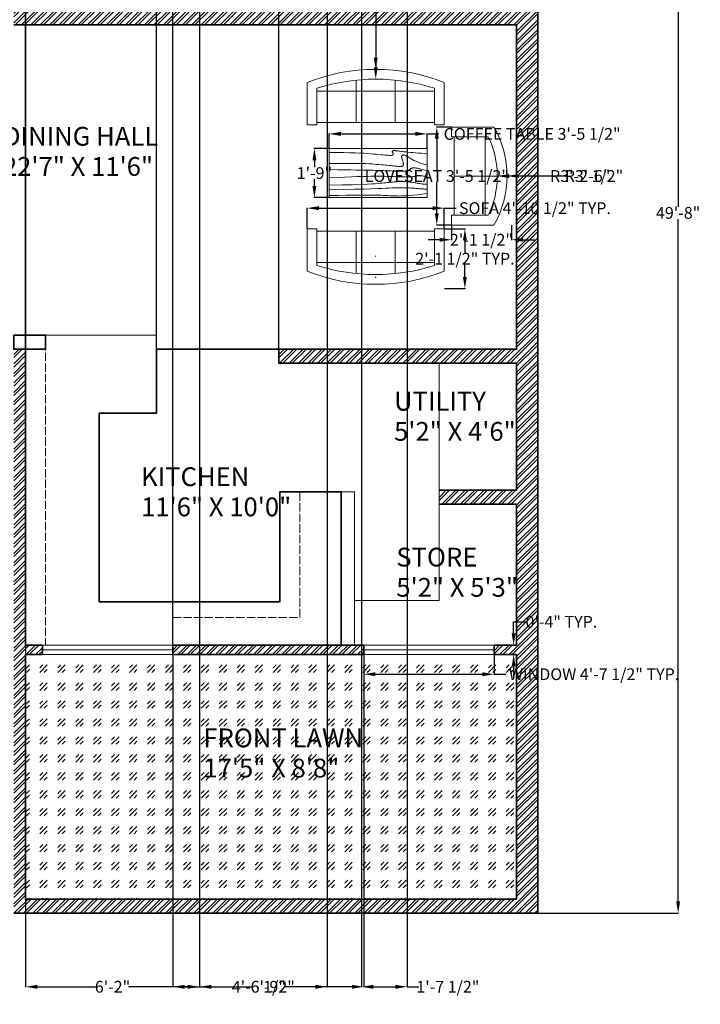
# Model space of a CAD drawing. Units: inches. Extents: x 334 to 846, y -424 to 250.
# Tile 2 of 3: x 557 to 846, y -424 to -5. Entities that reach past the tile are written whole.
import ezdxf

# ---------------------------------------------------------------- set-up
doc = ezdxf.new("R2010")
doc.units = ezdxf.units.IN
doc.header["$MEASUREMENT"] = 0
doc.linetypes.add('ACAD_ISO02W100', pattern=[15, 12, -3])
for name, color, linetype, lineweight in [('A-AREA-IDEN', 130, 'Continuous', 18), ('A-FLOR-FIXT', 8, 'Continuous', 18), ('A-FLOR-FIXT-HIDN', 8, 'ACAD_ISO02W100', 13), ('A-WALL', 7, 'Continuous', 35), ('A-WALL-PATT', 252, 'Continuous', 13), ('dimension', 130, 'Continuous', 18), ('furniture', 6, 'Continuous', 18), ('L-PLNT-PATT', 114, 'Continuous', 13), ('window', 150, 'Continuous', 18)]:
    doc.layers.add(name, color=color, linetype=linetype, lineweight=lineweight)
doc.styles.get("Standard").update_dxf_attribs({"font": 'arial.ttf'})
doc.dimstyles.get("Standard").update_dxf_attribs({"dimtxt": 5, "dimasz": 5, "dimexe": 0.18, "dimexo": 0.0625, "dimgap": 0.09, "dimtad": 0, "dimtih": 1, "dimtoh": 1, "dimdec": 1, "dimzin": 0, "dimdsep": 46, "dimlunit": 4, "dimtxsty": 'Standard', "dimcen": 0.09, "dimadec": 0, "dimazin": 0, "dimtfac": 1, "dimtdec": 1, "dimtofl": 0, "dimtmove": 0, "dimatfit": 3, "dimfxl": 1, "dimtolj": 1, "dimtzin": 0, "dimarcsym": 0})

# ---------------------------------------------------------------- blocks, each defined once
blk = doc.blocks.new('Sofa - Roundback 7 ft.')
for p, q in [((-36.000027, -34), (-36.000027, -11.4696)), ((-12.00002, -32.4421), (-12.00003, -6.5971)), ((11.99997, -32.4421), (11.99998, -6.5971)), ((35.99998, -34), (35.99998, -11.4696)), ((-35.999844, -13.3819), (35.9998, -13.3819)), ((-36.000027, -32.4421), (35.99998, -32.4421))]:
    blk.add_line(p, q)
for points in [[(-36.000027, -34), (-42.000027, -34), (-42.000027, -8)], [(41.99998, -8), (41.99998, -34), (35.99998, -34)]]:
    blk.add_lwpolyline(points)
for centre, radius, start, end in [((0, -114.25), 114.25, 68.43141, 111.5686), ((-0.00001, -127.1968), 121.1968, 72.72033, 107.2797)]:
    blk.add_arc(centre, radius, start, end)
blk = doc.blocks.new('Sofa - Roundback Loveseat 5 ft.')
for p, q in [((0, -32.44198), (0, -5.99998)), ((-24, -33.99998), (-24, -11.46958)), ((24.00004, -33.99998), (24.00004, -11.46958)), ((-23.9998, -13.38178), (23.99986, -13.38178)), ((-24, -32.44198), (24.00004, -32.44198))]:
    blk.add_line(p, q)
for points in [[(-24, -33.99998), (-30, -33.99998), (-30, -7.99998)], [(30.00004, -7.99998), (30.00004, -33.99998), (24.00004, -33.99998)]]:
    blk.add_lwpolyline(points)
for centre, radius, start, end in [((0, -60.24998), 60.24998, 60.13715, 119.8628), ((0, -61.38438), 55.38444, 64.32083, 115.6792)]:
    blk.add_arc(centre, radius, start, end)
blk = doc.blocks.new('Table - Rectangular Woodgrain 60 x 30 in.')
for p, q in [((0, 0), (0, -30)), ((60, 0), (0, 0)), ((60, -30), (60, 0)), ((0, -30), (60, -30))]:
    blk.add_line(p, q)
for points in [[(0, -2.4), (4.8155, -2.418), (9.0302, -2.4688), (12.709, -2.5477), (15.9167, -2.65), (18.7181, -2.7711), (21.1781, -2.9063), (23.3616, -3.0508), (25.3333, -3.2), (27.1477, -3.3495), (28.8172, -3.4958), (30.3437, -3.636), (31.7291, -3.7667), (32.9756, -3.8849), (34.0849, -3.9875), (35.059, -4.0714), (35.9, -4.1334), (36.6114, -4.1711), (37.2041, -4.1854), (37.6906, -4.1779), (38.0833, -4.15), (38.3948, -4.1034), (38.6375, -4.0396), (38.8239, -3.9602), (38.9666, -3.8667), (39.0764, -3.7608), (39.1573, -3.6448), (39.2116, -3.521), (39.2416, -3.3917), (39.2498, -3.2593), (39.2385, -3.1261), (39.21, -2.9944), (39.1666, -2.8667), (39.111, -2.7447), (39.0468, -2.6281), (38.978, -2.5163), (38.9083, -2.4083), (38.8418, -2.3035), (38.7823, -2.201), (38.7337, -2.1001), (38.7, -2), (38.6844, -1.9003), (38.6875, -1.8021), (38.7094, -1.707), (38.75, -1.6167), (38.8094, -1.5326), (38.8875, -1.4563), (38.9844, -1.3893), (39.1, -1.3333), (39.2351, -1.2896), (39.3937, -1.2583), (39.5804, -1.2396), (39.8, -1.2333), (40.057, -1.2396), (40.3562, -1.2583), (40.7023, -1.2896), (41.1, -1.3333), (41.5547, -1.3895), (42.0755, -1.4573), (42.6721, -1.5361), (43.3542, -1.625), (44.1316, -1.7233), (45.014, -1.8302), (46.0114, -1.9449), (47.1333, -2.0667), (48.3862, -2.1947), (49.7625, -2.3281), (51.2513, -2.4663), (52.8416, -2.6083), (54.5226, -2.7535), (56.2833, -2.9011), (58.1127, -3.0501), (60, -3.2)], [(0, -9.2), (6.5759, -9.0858), (11.9385, -9.0365), (16.2527, -9.0418), (19.6833, -9.0917), (22.3952, -9.1759), (24.5531, -9.2844), (26.322, -9.4069), (27.8666, -9.5333), (29.3241, -9.6553), (30.7203, -9.7719), (32.0532, -9.8837), (33.3208, -9.9917), (34.5213, -10.0965), (35.6526, -10.199), (36.7128, -10.2999), (37.7, -10.4), (38.6129, -10.4996), (39.4531, -10.5969), (40.223, -10.6895), (40.925, -10.775), (41.5613, -10.8512), (42.1344, -10.9156), (42.6465, -10.966), (43.1, -11), (43.4976, -11.0158), (43.8437, -11.0136), (44.143, -10.9942), (44.4, -10.9583), (44.6195, -10.9069), (44.8062, -10.8406), (44.9648, -10.7603), (45.1, -10.6667), (45.2155, -10.5598), (45.3114, -10.4365), (45.3871, -10.2929), (45.4416, -10.125), (45.4743, -9.929), (45.4844, -9.7011), (45.4709, -9.4371), (45.4333, -9.1333), (45.3716, -8.7883), (45.2896, -8.4104), (45.1919, -8.0107), (45.0833, -7.6), (44.9685, -7.1893), (44.8521, -6.7896), (44.7388, -6.4117), (44.6333, -6.0667), (44.54, -5.7628), (44.4614, -5.4979), (44.4001, -5.2675), (44.3583, -5.0667), (44.3384, -4.8909), (44.3427, -4.7354), (44.3736, -4.5956), (44.4333, -4.4667), (44.5236, -4.3453), (44.6427, -4.2333), (44.7884, -4.1339), (44.9583, -4.05), (45.1501, -3.9849), (45.3614, -3.9417), (45.59, -3.9234), (45.8333, -3.9333), (46.0915, -3.9749), (46.3734, -4.0531), (46.6906, -4.1736), (47.0542, -4.3417), (47.4756, -4.5629), (47.9661, -4.8427), (48.5372, -5.1866), (49.2, -5.6), (49.9676, -6.0844), (50.8594, -6.625), (51.8965, -7.2031), (53.1, -7.8), (54.491, -8.3969), (56.0906, -8.975), (57.9199, -9.5156), (60, -10)], [(0, -12.8), (5.1847, -12.9322), (9.6213, -13.0323), (13.3963, -13.1059), (16.5958, -13.1583), (19.3063, -13.1952), (21.614, -13.2219), (23.6054, -13.2439), (25.3666, -13.2667), (26.9728, -13.2947), (28.4531, -13.3281), (29.8256, -13.3663), (31.1083, -13.4083), (32.3191, -13.4535), (33.476, -13.501), (34.597, -13.5501), (35.7, -13.6), (36.7984, -13.6497), (37.8875, -13.6979), (38.9578, -13.743), (40, -13.7833), (41.0047, -13.8174), (41.9625, -13.8438), (42.864, -13.8607), (43.7, -13.8667), (44.4631, -13.8604), (45.1552, -13.8417), (45.7801, -13.8104), (46.3416, -13.7667), (46.8439, -13.7104), (47.2906, -13.6417), (47.6858, -13.5604), (48.0333, -13.4667), (48.3375, -13.3608), (48.6042, -13.2448), (48.8396, -13.121), (49.05, -12.9917), (49.2417, -12.8593), (49.4208, -12.7261), (49.5937, -12.5944), (49.7667, -12.4667), (49.9452, -12.3451), (50.1323, -12.2313), (50.3303, -12.1268), (50.5416, -12.0333), (50.7686, -11.9524), (51.0135, -11.8854), (51.2788, -11.8341), (51.5666, -11.8), (51.8785, -11.7843), (52.2116, -11.7865), (52.562, -11.8059), (52.926, -11.8417), (53.2998, -11.8931), (53.6795, -11.9594), (54.0614, -12.0397), (54.4416, -12.1333), (54.8223, -12.2401), (55.2293, -12.3625), (55.6942, -12.5037), (56.2489, -12.6667), (56.9251, -12.8547), (57.7545, -13.0708), (58.7689, -13.3182), (60, -13.6)], [(0, -18), (5.124, -17.7273), (9.6609, -17.5057), (13.6705, -17.3303), (17.2125, -17.1958), (20.3467, -17.0973), (23.1328, -17.0297), (25.6307, -16.9878), (27.9, -16.9667), (29.9928, -16.9617), (31.9302, -16.9703), (33.7254, -16.9907), (35.3917, -17.0208), (36.9423, -17.0588), (38.3906, -17.1026), (39.7499, -17.1503), (41.0333, -17.2), (42.2519, -17.2496), (43.4073, -17.2969), (44.4986, -17.3395), (45.525, -17.375), (46.4858, -17.4012), (47.3802, -17.4156), (48.2074, -17.416), (48.9667, -17.4), (49.6583, -17.3662), (50.2872, -17.3167), (50.8595, -17.2547), (51.3812, -17.1833), (51.8584, -17.1057), (52.2971, -17.025), (52.7034, -16.9443), (53.0833, -16.8667), (53.443, -16.7951), (53.789, -16.7313), (54.128, -16.6768), (54.4666, -16.6334), (54.8115, -16.6024), (55.1693, -16.5854), (55.5465, -16.5841), (55.95, -16.6), (56.3828, -16.6337), (56.8346, -16.6823), (57.2915, -16.7418), (57.7396, -16.8084), (58.165, -16.878), (58.5539, -16.9469), (58.8924, -17.0111), (59.1666, -17.0667), (59.3679, -17.1107), (59.5078, -17.1438), (59.6032, -17.1675), (59.6708, -17.1833), (59.7275, -17.193), (59.7901, -17.1979), (59.8753, -17.1998), (60, -17.2)], [(0, -22.4), (8.0098, -22.2501), (14.4094, -22.1011), (19.4168, -21.9535), (23.25, -21.8083), (26.1269, -21.6663), (28.2656, -21.5281), (29.884, -21.3947), (31.2, -21.2667), (32.3967, -21.1448), (33.5172, -21.0292), (34.5697, -20.9198), (35.5625, -20.8167), (36.5037, -20.7198), (37.4015, -20.6292), (38.2642, -20.5448), (39.1, -20.4667), (39.9164, -20.3951), (40.7187, -20.3313), (41.5117, -20.2768), (42.3, -20.2333), (43.0883, -20.2024), (43.8812, -20.1854), (44.6836, -20.1841), (45.5, -20.2), (46.3328, -20.234), (47.1747, -20.2844), (48.0163, -20.3488), (48.8479, -20.425), (49.66, -20.5106), (50.4429, -20.6031), (51.1872, -20.7004), (51.8833, -20.8), (52.5246, -20.8999), (53.1166, -20.9995), (53.6681, -21.0983), (54.1875, -21.1958), (54.6834, -21.2919), (55.1646, -21.3859), (55.6394, -21.4777), (56.1167, -21.5667), (56.6028, -21.6515), (57.0961, -21.7266), (57.5929, -21.7852), (58.0896, -21.8208), (58.5823, -21.8268), (59.0674, -21.7964), (59.5412, -21.723), (60, -21.6)], [(0, -25.2), (8.6355, -25.0504), (15.7026, -24.9031), (21.4049, -24.7606), (25.9458, -24.625), (29.529, -24.4988), (32.3578, -24.3844), (34.6359, -24.284), (36.5667, -24.2), (38.3213, -24.1341), (39.9417, -24.0854), (41.437, -24.0523), (42.8167, -24.0333), (44.0901, -24.0268), (45.2667, -24.0313), (46.3557, -24.0451), (47.3667, -24.0667), (48.309, -24.0947), (49.1928, -24.1287), (50.0284, -24.168), (50.826, -24.2125), (51.5959, -24.2617), (52.3483, -24.3151), (53.0935, -24.3725), (53.8417, -24.4334), (54.6009, -24.497), (55.3699, -24.561), (56.1454, -24.6226), (56.9239, -24.6792), (57.7021, -24.7279), (58.4764, -24.7662), (59.2435, -24.7911), (60, -24.8)], [(0, -28.8), (5.6867, -28.6681), (10.45, -28.5698), (14.407, -28.5012), (17.675, -28.4584), (20.3711, -28.4374), (22.6125, -28.4344), (24.5164, -28.4455), (26.2, -28.4667), (27.762, -28.4947), (29.2276, -28.5281), (30.6033, -28.5663), (31.8958, -28.6084), (33.1118, -28.6535), (34.2578, -28.7011), (35.3405, -28.7501), (36.3666, -28.8), (37.3443, -28.8497), (38.288, -28.8974), (39.2137, -28.9412), (40.1375, -28.9792), (41.0753, -29.0093), (42.0432, -29.0297), (43.0572, -29.0384), (44.1333, -29.0333), (45.2936, -29.0114), (46.5843, -28.9641), (48.0579, -28.8816), (49.7666, -28.7542), (51.7629, -28.5721), (54.0989, -28.3255), (56.8272, -28.0048), (60, -27.6)]]:
    blk.add_lwpolyline(points)
blk = doc.blocks.new('*D8')
at = {"layer": 'Defpoints', "color": 0, "ltscale": 0.3, "transparency": 16777216}
for p in [(777.06, 211), (777.06, -385), (836.82, -385)]:
    blk.add_point(p, dxfattribs=at)
at = {"layer": 'dimension', "color": 0, "lineweight": -2, "ltscale": 0.3, "transparency": 16777216}
for p, q in [((777.12, 211), (837, 211)), ((836.82, 206), (836.82, -84.36)), ((836.82, -380), (836.82, -89.65)), ((777.12, -385), (837, -385))]:
    blk.add_line(p, q, dxfattribs=at)
at = {"layer": 'dimension', "color": 0, "ltscale": 0.3, "transparency": 16777216}
for points in [[(835.99, 206), (837.66, 206), (836.82, 211)], [(835.99, -380), (837.66, -380), (836.82, -385)]]:
    blk.add_solid(points, dxfattribs=at)
at = {"layer": 'dimension', "color": 0, "ltscale": 0.3, "transparency": 16777216, "insert": (836.82, -87), "char_height": 5, "attachment_point": 5}
blk.add_mtext('\\A1;49\'-8"', dxfattribs=at)
blk = doc.blocks.new('WIN-55_5IN')
at = {"ltscale": 0.3}
blk.add_line((0, 2), (55.5, 2), dxfattribs=at)
blk.add_lwpolyline([(0, 4), (55.5, 4), (55.5, 0), (0, 0)], close=True, dxfattribs=at)
blk = doc.blocks.new('*D12')
at = {"layer": 'Defpoints', "color": 0, "ltscale": 0.3, "transparency": 16777216}
for p in [(737.3, -84.99), (678.9, -93.75), (737.3, -93.75)]:
    blk.add_point(p, dxfattribs=at)
at = {"layer": 'dimension', "color": 0, "lineweight": -2, "ltscale": 0.3, "transparency": 16777216}
for p, q in [((678.9, -93.69), (678.9, -84.81)), ((683.9, -84.99), (732.3, -84.99)), ((737.3, -93.69), (737.3, -84.81)), ((737.3, -84.99), (742.3, -84.99))]:
    blk.add_line(p, q, dxfattribs=at)
at = {"layer": 'dimension', "color": 0, "ltscale": 0.3, "transparency": 16777216}
for points in [[(683.9, -84.16), (683.9, -85.83), (678.9, -84.99)], [(732.3, -84.16), (732.3, -85.83), (737.3, -84.99)]]:
    blk.add_solid(points, dxfattribs=at)
at = {"layer": 'dimension', "color": 0, "ltscale": 0.3, "transparency": 16777216, "insert": (775.86, -84.99), "char_height": 5, "attachment_point": 5}
blk.add_mtext('\\A1;SOFA 4\'-10 1/2" TYP.', dxfattribs=at)
blk = doc.blocks.new('*D13')
at = {"layer": 'Defpoints', "color": 0, "ltscale": 0.3, "transparency": 16777216}
for p in [(737.3, -93.75), (737.3, -119.24), (746.06, -119.24)]:
    blk.add_point(p, dxfattribs=at)
at = {"layer": 'dimension', "color": 0, "lineweight": -2, "ltscale": 0.3, "transparency": 16777216}
for p, q in [((737.36, -93.75), (746.24, -93.75)), ((746.06, -98.75), (746.06, -103.82)), ((746.06, -114.24), (746.06, -109.17)), ((737.36, -119.24), (746.24, -119.24))]:
    blk.add_line(p, q, dxfattribs=at)
at = {"layer": 'dimension', "color": 0, "ltscale": 0.3, "transparency": 16777216}
for points in [[(745.22, -98.75), (746.89, -98.75), (746.06, -93.75)], [(745.22, -114.24), (746.89, -114.24), (746.06, -119.24)]]:
    blk.add_solid(points, dxfattribs=at)
at = {"layer": 'dimension', "color": 0, "ltscale": 0.3, "transparency": 16777216, "insert": (746.06, -106.5), "char_height": 5, "attachment_point": 5}
blk.add_mtext('\\A1;2\'-1 1/2" TYP.', dxfattribs=at)
blk = doc.blocks.new('*D14')
at = {"layer": 'Defpoints', "color": 0, "ltscale": 0.3, "transparency": 16777216}
for p in [(740.35, -50.46), (734.09, -92.17), (740.35, -92.17)]:
    blk.add_point(p, dxfattribs=at)
at = {"layer": 'dimension', "color": 0, "lineweight": -2, "ltscale": 0.3, "transparency": 16777216}
for p, q in [((740.29, -50.46), (733.91, -50.46)), ((734.09, -55.46), (734.09, -68.64)), ((734.09, -87.17), (734.09, -73.99)), ((740.29, -92.17), (733.91, -92.17))]:
    blk.add_line(p, q, dxfattribs=at)
at = {"layer": 'dimension', "color": 0, "ltscale": 0.3, "transparency": 16777216}
for points in [[(733.26, -55.46), (734.93, -55.46), (734.09, -50.46)], [(733.26, -87.17), (734.93, -87.17), (734.09, -92.17)]]:
    blk.add_solid(points, dxfattribs=at)
at = {"layer": 'dimension', "color": 0, "ltscale": 0.3, "transparency": 16777216, "insert": (734.09, -71.31), "char_height": 5, "attachment_point": 5}
blk.add_mtext('\\A1;LOVESEAT 3\'-5 1/2"', dxfattribs=at)
blk = doc.blocks.new('*D15')
at = {"layer": 'Defpoints', "color": 0, "ltscale": 0.3, "transparency": 16777216}
for p in [(740.35, -92.17), (765.84, -92.17), (765.84, -98.43)]:
    blk.add_point(p, dxfattribs=at)
at = {"layer": 'dimension', "color": 0, "lineweight": -2, "ltscale": 0.3, "transparency": 16777216}
for p, q in [((740.35, -92.23), (740.35, -98.61)), ((765.84, -92.23), (765.84, -98.61)), ((735.35, -98.43), (730.35, -98.43)), ((770.84, -98.43), (775.84, -98.43))]:
    blk.add_line(p, q, dxfattribs=at)
at = {"layer": 'dimension', "color": 0, "ltscale": 0.3, "transparency": 16777216}
for points in [[(735.35, -97.59), (735.35, -99.26), (740.35, -98.43)], [(770.84, -97.59), (770.84, -99.26), (765.84, -98.43)]]:
    blk.add_solid(points, dxfattribs=at)
at = {"layer": 'dimension', "color": 0, "ltscale": 0.3, "transparency": 16777216, "insert": (753.1, -98.43), "char_height": 5, "attachment_point": 5}
blk.add_mtext('\\A1;2\'-1 1/2"', dxfattribs=at)
blk = doc.blocks.new('*D16')
at = {"layer": 'Defpoints', "color": 0, "ltscale": 0.3, "transparency": 16777216}
for p in [(729.96, -53.38), (688.25, -59.63), (729.96, -59.63)]:
    blk.add_point(p, dxfattribs=at)
at = {"layer": 'dimension', "color": 0, "lineweight": -2, "ltscale": 0.3, "transparency": 16777216}
for p, q in [((688.25, -59.57), (688.25, -53.2)), ((693.25, -53.38), (724.96, -53.38)), ((729.96, -59.57), (729.96, -53.2)), ((729.96, -53.38), (734.96, -53.38))]:
    blk.add_line(p, q, dxfattribs=at)
at = {"layer": 'dimension', "color": 0, "ltscale": 0.3, "transparency": 16777216}
for points in [[(693.25, -52.54), (693.25, -54.21), (688.25, -53.38)], [(724.96, -52.54), (724.96, -54.21), (729.96, -53.38)]]:
    blk.add_solid(points, dxfattribs=at)
at = {"layer": 'dimension', "color": 0, "ltscale": 0.3, "transparency": 16777216, "insert": (774.67, -53.38), "char_height": 5, "attachment_point": 5}
blk.add_mtext('\\A1;COFFEE TABLE 3\'-5 1/2"', dxfattribs=at)
blk = doc.blocks.new('*D17')
at = {"layer": 'Defpoints', "color": 0, "ltscale": 0.3, "transparency": 16777216}
for p in [(682, -59.63), (688.25, -59.63), (688.25, -80.49)]:
    blk.add_point(p, dxfattribs=at)
at = {"layer": 'dimension', "color": 0, "lineweight": -2, "ltscale": 0.3, "transparency": 16777216}
for p, q in [((688.19, -59.63), (681.82, -59.63)), ((682, -64.63), (682, -67.42)), ((682, -75.49), (682, -72.7)), ((688.19, -80.49), (681.82, -80.49))]:
    blk.add_line(p, q, dxfattribs=at)
at = {"layer": 'dimension', "color": 0, "ltscale": 0.3, "transparency": 16777216}
for points in [[(681.16, -64.63), (682.83, -64.63), (682, -59.63)], [(681.16, -75.49), (682.83, -75.49), (682, -80.49)]]:
    blk.add_solid(points, dxfattribs=at)
at = {"layer": 'dimension', "color": 0, "ltscale": 0.3, "transparency": 16777216, "insert": (682, -70.06), "char_height": 5, "attachment_point": 5}
blk.add_mtext('\\A1;1\'-9"', dxfattribs=at)
blk = doc.blocks.new('*D18')
at = {"layer": 'Defpoints', "color": 0, "ltscale": 0.3, "transparency": 16777216}
for p in [(702.98, -275), (758.48, -275), (758.48, -283.33)]:
    blk.add_point(p, dxfattribs=at)
at = {"layer": 'dimension', "color": 0, "lineweight": -2, "ltscale": 0.3, "transparency": 16777216}
for p, q in [((702.98, -275.07), (702.98, -283.51)), ((758.48, -275.07), (758.48, -283.51)), ((707.98, -283.33), (753.48, -283.33)), ((758.48, -283.33), (763.48, -283.33))]:
    blk.add_line(p, q, dxfattribs=at)
at = {"layer": 'dimension', "color": 0, "ltscale": 0.3, "transparency": 16777216}
for points in [[(707.98, -282.5), (707.98, -284.16), (702.98, -283.33)], [(753.48, -282.5), (753.48, -284.16), (758.48, -283.33)]]:
    blk.add_solid(points, dxfattribs=at)
at = {"layer": 'dimension', "color": 0, "ltscale": 0.3, "transparency": 16777216, "insert": (801.03, -283.33), "char_height": 5, "attachment_point": 5}
blk.add_mtext('\\A1;WINDOW 4\'-7 1/2" TYP.', dxfattribs=at)
blk = doc.blocks.new('*D19')
at = {"layer": 'Defpoints', "color": 0, "ltscale": 0.3, "transparency": 16777216}
for p in [(758.48, -271), (766.8, -271), (758.48, -275)]:
    blk.add_point(p, dxfattribs=at)
at = {"layer": 'dimension', "color": 0, "lineweight": -2, "ltscale": 0.3, "transparency": 16777216}
for p, q in [((766.8, -266), (766.8, -261)), ((766.8, -261), (771.8, -261)), ((758.54, -271), (766.98, -271)), ((758.54, -275), (766.98, -275)), ((766.8, -280), (766.8, -285))]:
    blk.add_line(p, q, dxfattribs=at)
at = {"layer": 'dimension', "color": 0, "ltscale": 0.3, "transparency": 16777216}
for points in [[(765.97, -266), (767.64, -266), (766.8, -271)], [(765.97, -280), (767.64, -280), (766.8, -275)]]:
    blk.add_solid(points, dxfattribs=at)
at = {"layer": 'dimension', "color": 0, "ltscale": 0.3, "transparency": 16777216, "insert": (787.13, -261), "char_height": 5, "attachment_point": 5}
blk.add_mtext('\\A1;0\'-4" TYP.', dxfattribs=at)
blk = doc.blocks.new('*D20')
at = {"layer": 'Defpoints', "color": 0, "ltscale": 0.3, "transparency": 16777216}
for p in [(559.06, 149), (633.1, 149), (633.1, -416.35)]:
    blk.add_point(p, dxfattribs=at)
at = {"layer": 'dimension', "color": 0, "lineweight": -2, "ltscale": 0.3, "transparency": 16777216}
for p, q in [((559.06, 148.93), (559.06, -416.53)), ((633.1, 148.93), (633.1, -416.53)), ((564.06, -416.35), (589.33, -416.35)), ((628.1, -416.35), (602.83, -416.35))]:
    blk.add_line(p, q, dxfattribs=at)
at = {"layer": 'dimension', "color": 0, "ltscale": 0.3, "transparency": 16777216}
for points in [[(564.06, -415.52), (564.06, -417.19), (559.06, -416.35)], [(628.1, -415.52), (628.1, -417.19), (633.1, -416.35)]]:
    blk.add_solid(points, dxfattribs=at)
at = {"layer": 'dimension', "color": 0, "ltscale": 0.3, "transparency": 16777216, "insert": (596.08, -416.35), "char_height": 5, "attachment_point": 5}
blk.add_mtext('\\A1;6\'-2"', dxfattribs=at)
blk = doc.blocks.new('*D21')
at = {"layer": 'Defpoints', "color": 0, "ltscale": 0.3, "transparency": 16777216}
for p in [(633.1, 149), (687.41, 149), (687.41, -416.35)]:
    blk.add_point(p, dxfattribs=at)
at = {"layer": 'dimension', "color": 0, "lineweight": -2, "ltscale": 0.3, "transparency": 16777216}
for p, q in [((633.1, 148.93), (633.1, -416.53)), ((687.41, 148.93), (687.41, -416.53)), ((638.1, -416.35), (647.59, -416.35)), ((682.41, -416.35), (672.92, -416.35))]:
    blk.add_line(p, q, dxfattribs=at)
at = {"layer": 'dimension', "color": 0, "ltscale": 0.3, "transparency": 16777216}
for points in [[(638.1, -415.52), (638.1, -417.19), (633.1, -416.35)], [(682.41, -415.52), (682.41, -417.19), (687.41, -416.35)]]:
    blk.add_solid(points, dxfattribs=at)
at = {"layer": 'dimension', "color": 0, "ltscale": 0.3, "transparency": 16777216, "insert": (660.26, -416.35), "char_height": 5, "attachment_point": 5}
blk.add_mtext('\\A1;4\'-6 1/2"', dxfattribs=at)
blk = doc.blocks.new('*D22')
at = {"layer": 'Defpoints', "color": 0, "ltscale": 0.3, "transparency": 16777216}
for p in [(702.06, 149), (721.47, 149), (721.47, -416.35)]:
    blk.add_point(p, dxfattribs=at)
at = {"layer": 'dimension', "color": 0, "lineweight": -2, "ltscale": 0.3, "transparency": 16777216}
for p, q in [((702.06, 148.93), (702.06, -416.53)), ((721.47, 148.93), (721.47, -416.53)), ((707.06, -416.35), (716.47, -416.35)), ((721.47, -416.35), (726.47, -416.35))]:
    blk.add_line(p, q, dxfattribs=at)
at = {"layer": 'dimension', "color": 0, "ltscale": 0.3, "transparency": 16777216}
for points in [[(707.06, -415.52), (707.06, -417.19), (702.06, -416.35)], [(716.47, -415.52), (716.47, -417.19), (721.47, -416.35)]]:
    blk.add_solid(points, dxfattribs=at)
at = {"layer": 'dimension', "color": 0, "ltscale": 0.3, "transparency": 16777216, "insert": (738.8, -416.35), "char_height": 5, "attachment_point": 5}
blk.add_mtext('\\A1;1\'-7 1/2"', dxfattribs=at)
blk = doc.blocks.new('*D28')
at = {"layer": 'Defpoints', "color": 0, "ltscale": 0.3, "transparency": 16777216}
for p in [(666.86, 242.35), (614.79, -145), (666.86, -145)]:
    blk.add_point(p, dxfattribs=at)
at = {"layer": 'dimension', "color": 0, "lineweight": -2, "ltscale": 0.3, "transparency": 16777216}
for p, q in [((614.79, -144.94), (614.79, 242.53)), ((619.79, 242.35), (633.99, 242.35)), ((661.86, 242.35), (647.66, 242.35)), ((666.86, -144.94), (666.86, 242.53))]:
    blk.add_line(p, q, dxfattribs=at)
at = {"layer": 'dimension', "color": 0, "ltscale": 0.3, "transparency": 16777216}
for points in [[(619.79, 243.18), (619.79, 241.51), (614.79, 242.35)], [(661.86, 243.18), (661.86, 241.51), (666.86, 242.35)]]:
    blk.add_solid(points, dxfattribs=at)
at = {"layer": 'dimension', "color": 0, "ltscale": 0.3, "transparency": 16777216, "insert": (640.83, 242.35), "char_height": 5, "attachment_point": 5}
blk.add_mtext('\\A1;4\'-4"', dxfattribs=at)
blk = doc.blocks.new('*D29')
at = {"layer": 'Defpoints', "color": 0, "ltscale": 0.3, "transparency": 16777216}
for p in [(621.73, -275), (702.98, -275), (702.98, -416.35)]:
    blk.add_point(p, dxfattribs=at)
at = {"layer": 'dimension', "color": 0, "lineweight": -2, "ltscale": 0.3, "transparency": 16777216}
for p, q in [((621.73, -275.07), (621.73, -416.53)), ((702.98, -275.07), (702.98, -416.53)), ((626.73, -416.35), (655.6, -416.35)), ((697.98, -416.35), (669.1, -416.35))]:
    blk.add_line(p, q, dxfattribs=at)
at = {"layer": 'dimension', "color": 0, "ltscale": 0.3, "transparency": 16777216}
for points in [[(626.73, -415.52), (626.73, -417.19), (621.73, -416.35)], [(697.98, -415.52), (697.98, -417.19), (702.98, -416.35)]]:
    blk.add_solid(points, dxfattribs=at)
at = {"layer": 'dimension', "color": 0, "ltscale": 0.3, "transparency": 16777216, "insert": (662.35, -416.35), "char_height": 5, "attachment_point": 5}
blk.add_mtext('\\A1;6\'-9"', dxfattribs=at)
blk = doc.blocks.new('*D30')
at = {"layer": 'Defpoints', "color": 0, "ltscale": 0.3, "transparency": 16777216}
for p in [(621.73, 242.35), (559.06, -271), (621.73, -271)]:
    blk.add_point(p, dxfattribs=at)
at = {"layer": 'dimension', "color": 0, "lineweight": -2, "ltscale": 0.3, "transparency": 16777216}
for p, q in [((559.06, -270.94), (559.06, 242.53)), ((564.06, 242.35), (577.83, 242.35)), ((616.73, 242.35), (602.96, 242.35)), ((621.73, -270.94), (621.73, 242.53))]:
    blk.add_line(p, q, dxfattribs=at)
at = {"layer": 'dimension', "color": 0, "ltscale": 0.3, "transparency": 16777216}
for points in [[(564.06, 243.18), (564.06, 241.51), (559.06, 242.35)], [(616.73, 243.18), (616.73, 241.51), (621.73, 242.35)]]:
    blk.add_solid(points, dxfattribs=at)
at = {"layer": 'dimension', "color": 0, "ltscale": 0.3, "transparency": 16777216, "insert": (590.4, 242.35), "char_height": 5, "attachment_point": 5}
blk.add_mtext('\\A1;5\'-2 1/2"', dxfattribs=at)
blk = doc.blocks.new('*D34')
at = {"layer": 'Defpoints', "color": 0, "ltscale": 0.3, "transparency": 16777216}
for p in [(708.1, -30.1), (708.1, -114.35)]:
    blk.add_point(p, dxfattribs=at)
at = {"layer": 'dimension', "color": 0, "lineweight": -2, "ltscale": 0.3, "transparency": 16777216}
for p, q in [((713.1, 20.45), (708.1, 20.45)), ((708.1, 20.45), (708.1, -25.1)), ((708.01, -114.35), (708.19, -114.35)), ((708.1, -114.44), (708.1, -114.26))]:
    blk.add_line(p, q, dxfattribs=at)
at = {"layer": 'dimension', "color": 0, "ltscale": 0.3, "transparency": 16777216}
blk.add_solid([(707.27, -25.1), (708.93, -25.1), (708.1, -30.1)], dxfattribs=at)
at = {"layer": 'dimension', "color": 0, "ltscale": 0.3, "transparency": 16777216, "insert": (733.47, 20.45), "char_height": 5, "attachment_point": 5}
blk.add_mtext('\\A1;2X R7\'-0 1/2"', dxfattribs=at)
blk = doc.blocks.new('*D35')
at = {"layer": 'Defpoints', "color": 0, "ltscale": 0.3, "transparency": 16777216}
for p in [(708.1, -25.93), (708.1, -105.35)]:
    blk.add_point(p, dxfattribs=at)
at = {"layer": 'dimension', "color": 0, "lineweight": -2, "ltscale": 0.3, "transparency": 16777216}
for p, q in [((713.1, 21.73), (708.1, 21.73)), ((708.1, 21.73), (708.1, -20.93)), ((708.01, -105.35), (708.19, -105.35)), ((708.1, -105.44), (708.1, -105.26))]:
    blk.add_line(p, q, dxfattribs=at)
at = {"layer": 'dimension', "color": 0, "ltscale": 0.3, "transparency": 16777216}
blk.add_solid([(707.27, -20.93), (708.93, -20.93), (708.1, -25.93)], dxfattribs=at)
at = {"layer": 'dimension', "color": 0, "ltscale": 0.3, "transparency": 16777216, "insert": (733.47, 21.73), "char_height": 5, "attachment_point": 5}
blk.add_mtext('\\A1;2X R6\'-7 1/2"', dxfattribs=at)
blk = doc.blocks.new('*D36')
at = {"layer": 'Defpoints', "color": 0, "ltscale": 0.3, "transparency": 16777216}
for p in [(722.1, -71.31), (763.99, -71.31)]:
    blk.add_point(p, dxfattribs=at)
at = {"layer": 'dimension', "color": 0, "lineweight": -2, "ltscale": 0.3, "transparency": 16777216}
for p, q in [((722.1, -71.4), (722.1, -71.22)), ((722.01, -71.31), (722.19, -71.31)), ((789.12, -71.31), (768.99, -71.31))]:
    blk.add_line(p, q, dxfattribs=at)
at = {"layer": 'dimension', "color": 0, "ltscale": 0.3, "transparency": 16777216}
blk.add_solid([(768.99, -70.48), (768.99, -72.15), (763.99, -71.31)], dxfattribs=at)
at = {"layer": 'dimension', "color": 0, "ltscale": 0.3, "transparency": 16777216, "insert": (798.25, -71.31), "char_height": 5, "attachment_point": 5}
blk.add_mtext('\\A1;R3\'-6"', dxfattribs=at)
blk = doc.blocks.new('*D37')
at = {"layer": 'Defpoints', "color": 0, "ltscale": 0.3, "transparency": 16777216}
for p in [(721.31, -71.31), (759.82, -71.31)]:
    blk.add_point(p, dxfattribs=at)
at = {"layer": 'dimension', "color": 0, "lineweight": -2, "ltscale": 0.3, "transparency": 16777216}
for p, q in [((721.31, -71.4), (721.31, -71.22)), ((721.22, -71.31), (721.4, -71.31)), ((782.92, -71.31), (764.82, -71.31))]:
    blk.add_line(p, q, dxfattribs=at)
at = {"layer": 'dimension', "color": 0, "ltscale": 0.3, "transparency": 16777216}
blk.add_solid([(764.82, -70.48), (764.82, -72.15), (759.82, -71.31)], dxfattribs=at)
at = {"layer": 'dimension', "color": 0, "ltscale": 0.3, "transparency": 16777216, "insert": (797.87, -71.31), "char_height": 5, "attachment_point": 5}
blk.add_mtext('\\A1;R3\'-2 1/2"', dxfattribs=at)

msp = doc.modelspace()

# ---------------------------------------------------------------- hatches: boundary and pattern name
at = {"layer": 'A-WALL-PATT', "ltscale": 0.3}
h = msp.add_hatch(dxfattribs=at)
h.set_pattern_fill('ANSI32', color=256, scale=7.6)
h.paths.add_polyline_path([(559.06, 149), (633.1, 149), (633.1, 154), (559.06, 154), (554.06, 154), (554.06, 33.31), (559.06, 33.31)], flags=17)
h.paths.add_polyline_path([(777.06, 211), (380.06, 211), (380.06, -385), (389.06, -385), (389.06, -7), (490.06, -7), (490.06, -108.26), (496.06, -108.26), (496.06, -7), (496.06, -1), (389.06, -1), (389.06, 65), (493.06, 65), (493.06, 33.31), (496.06, 33.31), (496.06, 65), (518.06, 65), (518.06, 70), (389.06, 70), (389.06, 202), (554.06, 202), (562.49, 202), (768.06, 202), (768.06, 154), (721.47, 154), (721.47, 149), (768.06, 149), (768.06, -1), (702.06, -1), (702.06, 19.69), (697.06, 19.69), (697.06, -1), (554.06, -1), (554.06, -7), (697.06, -7), (768.06, -7), (768.06, -145), (702.06, -145), (697.06, -145), (666.86, -145), (666.86, -151), (697.06, -151), (702.06, -151), (768.06, -151), (768.06, -205), (735.06, -205), (735.06, -211), (768.06, -211), (768.06, -271), (758.48, -271), (758.48, -275), (768.06, -275), (768.06, -349), (768.06, -379), (702.06, -379), (697.06, -379), (559.06, -379), (559.06, -349), (559.06, -275), (566.23, -275), (566.23, -271), (559.06, -271), (559.06, -145), (554.06, -145), (554.06, -349), (554.06, -385), (559.06, -385), (697.06, -385), (702.06, -385), (768.06, -385), (777.06, -385), (777.06, -349)])
h = msp.add_hatch(dxfattribs=at)
h.set_pattern_fill('ANSI32', color=256, scale=7.6)
h.paths.add_polyline_path([(702.06, 154), (687.41, 154), (687.41, 149), (697.06, 149), (697.06, 56.25), (702.06, 56.25)], flags=17)
h.paths.add_polyline_path([(442.56, -139), (413.06, -139), (413.06, -145), (442.56, -145)], flags=17)
h.paths.add_polyline_path([(496.06, -139), (482.97, -139), (482.97, -145), (496.06, -145)], flags=17)
h.paths.add_polyline_path([(702.98, -271), (668.71, -271), (642.67, -271), (621.73, -271), (621.73, -275), (642.67, -275), (679.56, -275), (702.98, -275)], flags=17)
h.paths.add_polyline_path([(768.06, 63), (729.58, 63), (729.58, 59), (747.32, 59), (768.06, 59)], flags=17)
at = {"layer": 'L-PLNT-PATT', "ltscale": 0.3}
h = msp.add_hatch(dxfattribs=at)
h.set_pattern_fill('GOST_GLASS', color=256, scale=0.9)
h.set_pattern_definition([(45, (0, 0), (7.636753, 0), [4.5, -6.3]), (45, (1.909, 0), (7.636753, 0), [1.8, -9]), (45, (0, 1.909), (7.636753, 0), [1.8, -9])])
h.paths.add_polyline_path([(768.06, -275), (758.48, -275), (702.98, -275), (679.56, -275), (642.67, -275), (621.73, -275), (566.23, -275), (559.06, -275), (559.06, -349), (559.06, -379), (697.06, -379), (702.06, -379), (768.06, -379), (768.06, -349)])

# ---------------------------------------------------------------- linework, layer by layer
at = {"layer": 'A-FLOR-FIXT', "ltscale": 0.3}
for points in [[(567.61, -139), (600.4, -139), (614.79, -139), (614.79, -145)], [(735.06, -151), (735.06, -252), (699.21, -252)], [(699.02, -271), (699.02, -205.72), (693.33, -205.72)]]:
    msp.add_lwpolyline(points, dxfattribs=at)
at = {"layer": 'A-FLOR-FIXT-HIDN', "ltscale": 0.3}
for p, q in [((567.61, -142), (567.61, -271)), ((675.81, -259.13), (675.81, -205.72)), ((621.73, -271), (621.73, -259.13)), ((621.73, -259.13), (675.81, -259.13))]:
    msp.add_line(p, q, dxfattribs=at)
at = {"layer": 'A-WALL'}
for p, q in [((559.06, -145), (559.06, -271)), ((768.06, -211), (768.06, -271)), ((559.06, -275), (559.06, -349)), ((768.06, -275), (768.06, -349))]:
    msp.add_line(p, q, dxfattribs=at)
at = {"layer": 'A-WALL', "ltscale": 0.3}
for p, q in [((735.06, -211), (768.06, -211)), ((566.23, -271), (566.23, -275)), ((758.48, -271), (758.48, -275)), ((758.48, -271), (768.06, -271)), ((559.06, -349), (559.06, -379)), ((768.06, -349), (768.06, -379))]:
    msp.add_line(p, q, dxfattribs=at)
for points in [[(554.06, -385), (559.06, -385), (697.06, -385), (702.06, -385), (768.06, -385), (777.06, -385), (777.06, -349), (777.06, 211), (380.06, 211), (380.06, -385)], [(666.86, -145), (697.06, -145), (702.06, -145), (768.06, -145), (768.06, -7), (697.06, -7), (554.06, -7)], [(554.06, -145), (559.06, -145), (567.61, -145)], [(735.06, -205), (768.06, -205), (768.06, -151), (702.06, -151), (697.06, -151), (666.86, -151), (666.86, -145), (614.79, -145), (614.79, -172.27), (590.38, -172.27), (590.38, -252.49), (667.29, -252.49), (667.29, -205.72), (693.33, -205.72), (693.33, -271)], [(559.06, -271), (566.23, -271)], [(674.4, -271), (679.56, -271)], [(559.06, -275), (566.23, -275)], [(758.48, -275), (768.06, -275)], [(559.06, -379), (697.06, -379), (702.06, -379), (768.06, -379)]]:
    msp.add_lwpolyline(points, dxfattribs=at)
for points in [[(554.06, -139), (567.61, -139), (567.61, -145), (554.06, -145)], [(668.71, -271), (642.67, -271), (621.73, -271), (621.73, -275), (642.67, -275), (679.56, -275), (702.98, -275), (702.98, -271)]]:
    msp.add_lwpolyline(points, close=True, dxfattribs=at)

# ---------------------------------------------------------------- block references
at = {"layer": 'furniture', "ltscale": 0.3, "xscale": 0.6951845112935744, "yscale": 0.6951845112935744, "zscale": 0.6951845112935744}
for name, p in [('Sofa - Roundback 7 ft.', (708.1, -25.93)), ('Table - Rectangular Woodgrain 60 x 30 in.', (688.25, -59.63))]:
    msp.add_blockref(name, p, dxfattribs=at)
at = {"layer": 'furniture', "ltscale": 0.3, "yscale": 0.6951845112935744, "zscale": 0.6951845112935744}
for name, p, xscale, rotation in [('Sofa - Roundback Loveseat 5 ft.', (763.99, -71.31), 0.6951845112935744, 270), ('Sofa - Roundback 7 ft.', (708.1, -117.39), -0.6951845112935744, 180)]:
    msp.add_blockref(name, p, dxfattribs=dict(at, xscale=xscale, rotation=rotation))
at = {"layer": 'window'}
for p in [(566.23, -275), (702.98, -275)]:
    msp.add_blockref('WIN-55_5IN', p, dxfattribs=at)

# ---------------------------------------------------------------- texts
at = {"layer": 'A-AREA-IDEN', "ltscale": 0.3}
for s, p in [('DINING HALL', (549.43, -58.39)), ('22\'7" X 11\'6"', (549.43, -71.24)), ('UTILITY', (715.92, -171.14)), ('5\'2" X 4\'6"', (715.92, -183.99)), ('KITCHEN', (608.25, -203.27)), ('11\'6" X 10\'0"', (608.25, -216.12)), ('STORE', (716.86, -237.5)), ('5\'2" X 5\'3"', (716.86, -250.35)), ('FRONT LAWN', (634.76, -314.43)), ('17\'5" X 8\'8"', (634.76, -327.28))]:
    msp.add_text(s, height=8, dxfattribs=at).set_placement(p)

# ---------------------------------------------------------------- dimensions: what is measured, and where the dimension line sits
at = {"layer": 'dimension', "ltscale": 0.3}
for base, p1, p2, picture, middle in [((621.73, 242.35), (559.06, -271), (621.73, -271), '*D30', (590.4, 242.35)), ((666.86, 242.35), (614.79, -145), (666.86, -145), '*D28', (640.83, 242.35)), ((633.1, -416.35), (559.06, 149), (633.1, 149), '*D20', (596.08, -416.35)), ((687.41, -416.35), (633.1, 149), (687.41, 149), '*D21', (660.26, -416.35)), ((721.47, -416.35), (702.06, 149), (721.47, 149), '*D22', (738.8, -416.35)), ((765.84, -98.43), (740.35, -92.17), (765.84, -92.17), '*D15', (753.1, -98.43)), ((702.9767, -416.3541), (621.7296, -275.0041), (702.9767, -275.0041), '*D29', (662.3531, -416.3541))]:
    dim = msp.add_linear_dim(base=base, p1=p1, p2=p2, dimstyle='Standard', override={"dimdec": 1, "dimlfac": 1, "dimrnd": 0, "dimzin": 1, "dimdsep": 46, "dimlunit": 4, "dimfrac": 2}, dxfattribs=at)
    dim.commit()
    dim.dimension.update_dxf_attribs({"geometry": picture, "text_midpoint": middle})
for base, p1, p2, override, picture, middle in [((836.82, -385), (777.06, 211), (777.06, -385), {"dimclrd": 0, "dimclre": 0, "dimclrt": 0}, '*D8', (836.82, -87)), ((682, -59.63), (688.25, -80.49), (688.25, -59.63), {"dimdec": 1, "dimlfac": 1, "dimrnd": 0, "dimzin": 1, "dimdsep": 46, "dimlunit": 4, "dimfrac": 2}, '*D17', (682, -70.06))]:
    dim = msp.add_linear_dim(base=base, p1=p1, p2=p2, angle=90, dimstyle='Standard', override=override, dxfattribs=at)
    dim.commit()
    dim.dimension.update_dxf_attribs({"geometry": picture, "text_midpoint": middle})
for center, mpoint, picture, middle in [((708.1, -105.35), (708.1, -25.93), '*D35', (733.47, 21.73)), ((708.0998, -114.3517), (708.1, -30.0975), '*D34', (733.4681, 20.455))]:
    dim = msp.add_radius_dim(center=center, mpoint=mpoint, text='2X <>', dimstyle='Standard', override={"dimdec": 1, "dimlfac": 1, "dimrnd": 0, "dimzin": 1, "dimdsep": 46, "dimlunit": 4, "dimfrac": 2}, dxfattribs=at)
    dim.commit()
    dim.dimension.update_dxf_attribs({"geometry": picture, "text_midpoint": middle, "dimtype": 164})
for base, p1, p2, text, picture, middle in [((729.96, -53.38), (688.25, -59.63), (729.96, -59.63), 'COFFEE TABLE <>', '*D16', (774.67, -53.38)), ((737.3, -84.99), (678.9, -93.75), (737.3, -93.75), 'SOFA <> TYP.', '*D12', (775.86, -84.99)), ((758.48, -283.33), (702.98, -275), (758.48, -275), 'WINDOW <> TYP.', '*D18', (801.03, -283.33))]:
    dim = msp.add_linear_dim(base=base, p1=p1, p2=p2, text=text, dimstyle='Standard', override={"dimdec": 1, "dimlfac": 1, "dimrnd": 0, "dimzin": 1, "dimdsep": 46, "dimlunit": 4, "dimfrac": 2}, dxfattribs=at)
    dim.commit()
    dim.dimension.update_dxf_attribs({"geometry": picture, "text_midpoint": middle})
for base, p1, p2, angle, text, picture, middle in [((734.09, -92.17), (740.35, -50.46), (740.35, -92.17), 270, 'LOVESEAT <>', '*D14', (734.09, -71.31)), ((746.06, -119.24), (737.3, -93.75), (737.3, -119.24), 270, '<> TYP.', '*D13', (746.06, -106.5)), ((766.8, -271), (758.48, -275), (758.48, -271), 90, '<> TYP.', '*D19', (787.13, -261))]:
    dim = msp.add_linear_dim(base=base, p1=p1, p2=p2, angle=angle, text=text, dimstyle='Standard', override={"dimdec": 1, "dimlfac": 1, "dimrnd": 0, "dimzin": 1, "dimdsep": 46, "dimlunit": 4, "dimfrac": 2}, dxfattribs=at)
    dim.commit()
    dim.dimension.update_dxf_attribs({"geometry": picture, "text_midpoint": middle})
for center, mpoint, picture, middle in [((721.31, -71.31), (759.82, -71.31), '*D37', (782.92, -71.31)), ((722.1, -71.31), (763.99, -71.31), '*D36', (789.12, -71.31))]:
    dim = msp.add_radius_dim(center=center, mpoint=mpoint, dimstyle='Standard', override={"dimdec": 1, "dimlfac": 1, "dimrnd": 0, "dimzin": 1, "dimdsep": 46, "dimlunit": 4, "dimfrac": 2}, dxfattribs=at)
    dim.commit()
    dim.dimension.update_dxf_attribs({"geometry": picture, "text_midpoint": middle, "dimtype": 164})

doc.saveas('drawing.dxf')
